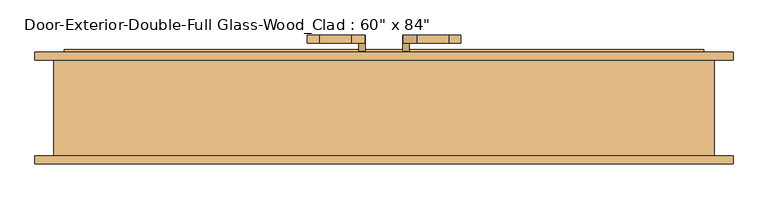
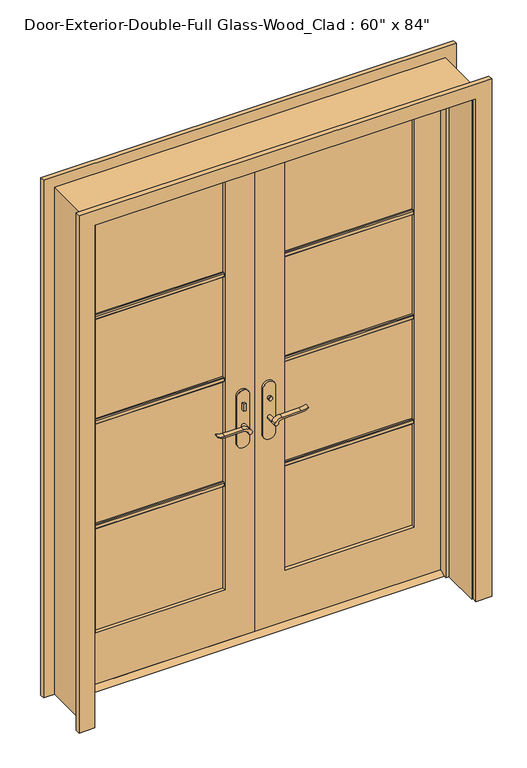
"""IFC4 building model written with IfcOpenShell, lengths in millimetres: door geometry."""

from ifc_helpers import new_model, si_unit, point, frame, frame_2d, origin, place, context, project, spatial, polyline, circle_curve, trimmed, segment, composite_curve, outline, extrude, faceted_brep, source, transform, mapped, element, save


def door_014e9f54(model_context):
    return source(origin(), model_context, "Body", "SolidModel", [
        extrude(outline(polyline([(76.2, 12.7), (111.125, 12.7), (136.525, 0.0), (50.8, 0.0), (76.2, 12.7)])), frame((-762.0, 0.0, 0.0), z_axis=(1.0, 0.0, 0.0), x_axis=(0.0, 1.0, 0.0)), (0.0, 0.0, 1.0), 1524.0),
        extrude(outline(polyline([(-47.4019111, 56.2), (-57.4019111, 56.2), (-57.4019111, 66.2), (-47.4019111, 66.2), (-47.4019111, 56.2)])), frame((0.0, 0.0, 981.9), z_axis=(0.0, 0.0, 1.0), x_axis=(1.0, 0.0, 0.0)), (0.0, 0.0, 1.0), 30.0),
        extrude(outline(composite_curve([segment(trimmed(circle_curve(frame_2d((996.9, -52.4019111)), 8.0), [point((996.9, -60.4019111))], [point((996.9, -44.4019111))], False, "CARTESIAN"), True, "CONTINUOUS"), segment(trimmed(circle_curve(frame_2d((996.9, -52.4019111)), 8.0), [point((996.9, -44.4019111))], [point((996.9, -60.4019111))], False, "CARTESIAN"), True, "CONTINUOUS")], self_intersect=False)), frame((0.0, 121.125, 0.0), z_axis=(0.0, 1.0, 0.0), x_axis=(0.0, 0.0, 1.0)), (0.0, 0.0, 1.0), 10.0),
        extrude(outline(composite_curve([segment(trimmed(circle_curve(frame_2d((897.1555521, -76.0694241)), 37.2832219), [point((919.0523287, -45.8937749))], [point((934.4, -77.7693445))], False, "CARTESIAN"), True, "CONTINUOUS"), segment(polyline([(934.4, -77.7693445), (934.4, -154.045502)]), True, "CONTINUOUS"), segment(trimmed(circle_curve(frame_2d((1017.6850638, -153.9791202)), 83.2850902), [point((934.4, -154.045502))], [point((939.4, -182.4019111))], True, "CARTESIAN"), True, "CONTINUOUS"), segment(polyline([(939.4, -182.4019111), (936.6135558, -182.4019111)]), True, "CONTINUOUS"), segment(trimmed(circle_curve(frame_2d((986.6709207, -150.4622499)), 59.3791355), [point((936.6135558, -182.4019111))], [point((927.4, -154.045502))], False, "CARTESIAN"), True, "CONTINUOUS"), segment(polyline([(927.4, -154.045502), (927.4, -77.7881013)]), True, "CONTINUOUS"), segment(trimmed(circle_curve(frame_2d((909.2738613, -77.7881013)), 18.1261387), [point((927.4, -77.7881013))], [point((914.4, -60.4019111))], True, "CARTESIAN"), True, "CONTINUOUS"), segment(trimmed(circle_curve(frame_2d((914.4, -52.4019111)), 8.0), [point((914.4, -60.4019111))], [point((919.0523287, -45.8937749))], False, "CARTESIAN"), True, "CONTINUOUS")], self_intersect=False)), frame((0.0, 16.2, 0.0), z_axis=(0.0, 1.0, 0.0), x_axis=(0.0, 0.0, 1.0)), (0.0, 0.0, 1.0), 20.0),
        extrude(outline(composite_curve([segment(trimmed(circle_curve(frame_2d((914.4, -52.4019111)), 8.0), [point((914.3999903, -60.4019111))], [point((919.0523287, -45.8937749))], False, "CARTESIAN"), True, "CONTINUOUS"), segment(trimmed(circle_curve(frame_2d((897.1555521, -76.0694241)), 37.2832219), [point((919.0523287, -45.8937749))], [point((934.4, -77.7693445))], False, "CARTESIAN"), True, "CONTINUOUS"), segment(polyline([(934.4, -77.7693445), (934.4, -154.045502)]), True, "CONTINUOUS"), segment(trimmed(circle_curve(frame_2d((1017.6850638, -153.9791202)), 83.2850902), [point((934.4, -154.045502))], [point((939.4, -182.4019111))], True, "CARTESIAN"), True, "CONTINUOUS"), segment(polyline([(939.4, -182.4019111), (936.6135558, -182.4019111)]), True, "CONTINUOUS"), segment(trimmed(circle_curve(frame_2d((986.6709207, -150.4622499)), 59.3791355), [point((936.6135558, -182.4019111))], [point((927.4, -154.045502))], False, "CARTESIAN"), True, "CONTINUOUS"), segment(polyline([(927.4, -154.045502), (927.4, -77.788099)]), True, "CONTINUOUS"), segment(trimmed(circle_curve(frame_2d((909.2738682, -77.788099)), 18.1261318), [point((927.4, -77.788099))], [point((914.3999903, -60.4019111))], True, "CARTESIAN"), True, "CONTINUOUS")], self_intersect=False)), frame((0.0, 151.125, 0.0), z_axis=(0.0, 1.0, 0.0), x_axis=(0.0, 0.0, 1.0)), (0.0, 0.0, 1.0), 20.0),
        extrude(outline(composite_curve([segment(trimmed(circle_curve(frame_2d((914.4, -52.4019111)), 8.0), [point((914.4, -60.4019111))], [point((914.4, -44.4019111))], False, "CARTESIAN"), True, "CONTINUOUS"), segment(trimmed(circle_curve(frame_2d((914.4, -52.4019111)), 8.0), [point((914.4, -44.4019111))], [point((914.4, -60.4019111))], False, "CARTESIAN"), True, "CONTINUOUS")], self_intersect=False)), frame((0.0, 36.2, 0.0), z_axis=(0.0, 1.0, 0.0), x_axis=(0.0, 0.0, 1.0)), (0.0, 0.0, 1.0), 30.0),
        extrude(outline(composite_curve([segment(trimmed(circle_curve(frame_2d((914.4, -52.4019111)), 8.0), [point((914.4, -60.4019111))], [point((914.4, -44.4019111))], False, "CARTESIAN"), True, "CONTINUOUS"), segment(trimmed(circle_curve(frame_2d((914.4, -52.4019111)), 8.0), [point((914.4, -44.4019111))], [point((914.4, -60.4019111))], False, "CARTESIAN"), True, "CONTINUOUS")], self_intersect=False)), frame((0.0, 121.125, 0.0), z_axis=(0.0, 1.0, 0.0), x_axis=(0.0, 0.0, 1.0)), (0.0, 0.0, 1.0), 30.0),
        extrude(outline(composite_curve([segment(polyline([(844.4, -27.4019111), (1039.4, -27.4019111)]), True, "CONTINUOUS"), segment(trimmed(circle_curve(frame_2d((1039.4, -52.4019111)), 25.0), [point((1039.4, -27.4019111))], [point((1039.4, -77.4019111))], False, "CARTESIAN"), True, "CONTINUOUS"), segment(polyline([(1039.4, -77.4019111), (844.4, -77.4019111)]), True, "CONTINUOUS"), segment(trimmed(circle_curve(frame_2d((844.4, -52.4019111)), 25.0), [point((844.4, -77.4019111))], [point((844.4, -27.4019111))], False, "CARTESIAN"), True, "CONTINUOUS")], self_intersect=False)), frame((0.0, 66.2, 0.0), z_axis=(0.0, 1.0, 0.0), x_axis=(0.0, 0.0, 1.0)), (0.0, 0.0, 1.0), 10.0),
        extrude(outline(composite_curve([segment(polyline([(844.4, -27.4019111), (1039.4, -27.4019111)]), True, "CONTINUOUS"), segment(trimmed(circle_curve(frame_2d((1039.4, -52.4019111)), 25.0), [point((1039.4, -27.4019111))], [point((1039.4, -77.4019111))], False, "CARTESIAN"), True, "CONTINUOUS"), segment(polyline([(1039.4, -77.4019111), (844.4, -77.4019111)]), True, "CONTINUOUS"), segment(trimmed(circle_curve(frame_2d((844.4, -52.4019111)), 25.0), [point((844.4, -77.4019111))], [point((844.4, -27.4019111))], False, "CARTESIAN"), True, "CONTINUOUS")], self_intersect=False)), frame((0.0, 111.125, 0.0), z_axis=(0.0, 1.0, 0.0), x_axis=(0.0, 0.0, 1.0)), (0.0, 0.0, 1.0), 10.0),
        extrude(outline(polyline([(47.3875, 131.125), (57.3875, 131.125), (57.3875, 121.125), (47.3875, 121.125), (47.3875, 131.125)])), frame((0.0, 0.0, 981.9), z_axis=(0.0, 0.0, 1.0), x_axis=(1.0, 0.0, 0.0)), (0.0, 0.0, 1.0), 30.0),
        extrude(outline(composite_curve([segment(trimmed(circle_curve(frame_2d((996.9, 52.3875)), 8.0), [point((996.9, 60.3875))], [point((996.9, 44.3875))], False, "CARTESIAN"), True, "CONTINUOUS"), segment(trimmed(circle_curve(frame_2d((996.9, 52.3875)), 8.0), [point((996.9, 44.3875))], [point((996.9, 60.3875))], False, "CARTESIAN"), True, "CONTINUOUS")], self_intersect=False)), frame((0.0, 56.2, 0.0), z_axis=(0.0, 1.0, 0.0), x_axis=(0.0, 0.0, 1.0)), (0.0, 0.0, 1.0), 10.0),
        extrude(outline(composite_curve([segment(trimmed(circle_curve(frame_2d((914.4, 52.3875)), 8.0), [point((919.0523287, 45.8793637))], [point((914.4, 60.3875))], False, "CARTESIAN"), True, "CONTINUOUS"), segment(trimmed(circle_curve(frame_2d((909.2738613, 77.7736901)), 18.1261387), [point((914.4, 60.3875))], [point((927.4, 77.7736901))], True, "CARTESIAN"), True, "CONTINUOUS"), segment(polyline([(927.4, 77.7736901), (927.4, 154.0310909)]), True, "CONTINUOUS"), segment(trimmed(circle_curve(frame_2d((986.6709207, 150.4478388)), 59.3791355), [point((927.4, 154.0310909))], [point((936.6135558, 182.3875))], False, "CARTESIAN"), True, "CONTINUOUS"), segment(polyline([(936.6135558, 182.3875), (939.4, 182.3875)]), True, "CONTINUOUS"), segment(trimmed(circle_curve(frame_2d((1017.6850638, 153.9647091)), 83.2850902), [point((939.4, 182.3875))], [point((934.4, 154.0310909))], True, "CARTESIAN"), True, "CONTINUOUS"), segment(polyline([(934.4, 154.0310909), (934.4, 77.7549333)]), True, "CONTINUOUS"), segment(trimmed(circle_curve(frame_2d((897.1555521, 76.0550129)), 37.2832219), [point((934.4, 77.7549333))], [point((919.0523287, 45.8793637))], False, "CARTESIAN"), True, "CONTINUOUS")], self_intersect=False)), frame((0.0, 151.125, 0.0), z_axis=(0.0, 1.0, 0.0), x_axis=(0.0, 0.0, 1.0)), (0.0, 0.0, 1.0), 20.0),
        extrude(outline(composite_curve([segment(trimmed(circle_curve(frame_2d((909.2738682, 77.7736878)), 18.1261318), [point((914.3999903, 60.3875))], [point((927.4, 77.7736878))], True, "CARTESIAN"), True, "CONTINUOUS"), segment(polyline([(927.4, 77.7736878), (927.4, 154.0310909)]), True, "CONTINUOUS"), segment(trimmed(circle_curve(frame_2d((986.6709207, 150.4478388)), 59.3791355), [point((927.4, 154.0310909))], [point((936.6135558, 182.3875))], False, "CARTESIAN"), True, "CONTINUOUS"), segment(polyline([(936.6135558, 182.3875), (939.4, 182.3875)]), True, "CONTINUOUS"), segment(trimmed(circle_curve(frame_2d((1017.6850638, 153.9647091)), 83.2850902), [point((939.4, 182.3875))], [point((934.4, 154.0310909))], True, "CARTESIAN"), True, "CONTINUOUS"), segment(polyline([(934.4, 154.0310909), (934.4, 77.7549333)]), True, "CONTINUOUS"), segment(trimmed(circle_curve(frame_2d((897.1555521, 76.0550129)), 37.2832219), [point((934.4, 77.7549333))], [point((919.0523287, 45.8793637))], False, "CARTESIAN"), True, "CONTINUOUS"), segment(trimmed(circle_curve(frame_2d((914.4, 52.3875)), 8.0), [point((919.0523287, 45.8793637))], [point((914.3999903, 60.3875))], False, "CARTESIAN"), True, "CONTINUOUS")], self_intersect=False)), frame((0.0, 16.2, 0.0), z_axis=(0.0, 1.0, 0.0), x_axis=(0.0, 0.0, 1.0)), (0.0, 0.0, 1.0), 20.0),
        extrude(outline(composite_curve([segment(trimmed(circle_curve(frame_2d((914.4, 52.3875)), 8.0), [point((914.4, 60.3875))], [point((914.4, 44.3875))], False, "CARTESIAN"), True, "CONTINUOUS"), segment(trimmed(circle_curve(frame_2d((914.4, 52.3875)), 8.0), [point((914.4, 44.3875))], [point((914.4, 60.3875))], False, "CARTESIAN"), True, "CONTINUOUS")], self_intersect=False)), frame((0.0, 121.125, 0.0), z_axis=(0.0, 1.0, 0.0), x_axis=(0.0, 0.0, 1.0)), (0.0, 0.0, 1.0), 30.0),
        extrude(outline(composite_curve([segment(trimmed(circle_curve(frame_2d((914.4, 52.3875)), 8.0), [point((914.4, 60.3875))], [point((914.4, 44.3875))], False, "CARTESIAN"), True, "CONTINUOUS"), segment(trimmed(circle_curve(frame_2d((914.4, 52.3875)), 8.0), [point((914.4, 44.3875))], [point((914.4, 60.3875))], False, "CARTESIAN"), True, "CONTINUOUS")], self_intersect=False)), frame((0.0, 36.2, 0.0), z_axis=(0.0, 1.0, 0.0), x_axis=(0.0, 0.0, 1.0)), (0.0, 0.0, 1.0), 30.0),
        extrude(outline(composite_curve([segment(trimmed(circle_curve(frame_2d((844.4, 52.3875)), 25.0), [point((844.4, 27.3875))], [point((844.4, 77.3875))], False, "CARTESIAN"), True, "CONTINUOUS"), segment(polyline([(844.4, 77.3875), (1039.4, 77.3875)]), True, "CONTINUOUS"), segment(trimmed(circle_curve(frame_2d((1039.4, 52.3875)), 25.0), [point((1039.4, 77.3875))], [point((1039.4, 27.3875))], False, "CARTESIAN"), True, "CONTINUOUS"), segment(polyline([(1039.4, 27.3875), (844.4, 27.3875)]), True, "CONTINUOUS")], self_intersect=False)), frame((0.0, 111.125, 0.0), z_axis=(0.0, 1.0, 0.0), x_axis=(0.0, 0.0, 1.0)), (0.0, 0.0, 1.0), 10.0),
        extrude(outline(composite_curve([segment(trimmed(circle_curve(frame_2d((844.4, 52.3875)), 25.0), [point((844.4, 27.3875))], [point((844.4, 77.3875))], False, "CARTESIAN"), True, "CONTINUOUS"), segment(polyline([(844.4, 77.3875), (1039.4, 77.3875)]), True, "CONTINUOUS"), segment(trimmed(circle_curve(frame_2d((1039.4, 52.3875)), 25.0), [point((1039.4, 77.3875))], [point((1039.4, 27.3875))], False, "CARTESIAN"), True, "CONTINUOUS"), segment(polyline([(1039.4, 27.3875), (844.4, 27.3875)]), True, "CONTINUOUS")], self_intersect=False)), frame((0.0, 66.2, 0.0), z_axis=(0.0, 1.0, 0.0), x_axis=(0.0, 0.0, 1.0)), (0.0, 0.0, 1.0), 10.0),
        extrude(outline(polyline([(90.17, 1578.371875), (90.17, 1559.321875), (83.82, 1559.321875), (80.645, 1562.496875), (80.645, 1575.196875), (83.82, 1578.371875), (90.17, 1578.371875)])), frame((120.65, 0.0, 0.0), z_axis=(1.0, 0.0, 0.0), x_axis=(0.0, 1.0, 0.0)), (0.0, 0.0, 1.0), 520.7),
        extrude(outline(polyline([(90.17, 1132.68125), (90.17, 1113.63125), (83.82, 1113.63125), (80.645, 1116.80625), (80.645, 1129.50625), (83.82, 1132.68125), (90.17, 1132.68125)])), frame((120.65, 0.0, 0.0), z_axis=(1.0, 0.0, 0.0), x_axis=(0.0, 1.0, 0.0)), (0.0, 0.0, 1.0), 520.7),
        extrude(outline(polyline([(90.17, 686.990625), (90.17, 667.940625), (83.82, 667.940625), (80.645, 671.115625), (80.645, 683.815625), (83.82, 686.990625), (90.17, 686.990625)])), frame((120.65, 0.0, 0.0), z_axis=(1.0, 0.0, 0.0), x_axis=(0.0, 1.0, 0.0)), (0.0, 0.0, 1.0), 520.7),
        extrude(outline(polyline([(97.155, 1578.371875), (103.505, 1578.371875), (106.68, 1575.196875), (106.68, 1562.496875), (103.505, 1559.321875), (97.155, 1559.321875), (97.155, 1578.371875)])), frame((-641.35, 0.0, 0.0), z_axis=(1.0, 0.0, 0.0), x_axis=(0.0, 1.0, 0.0)), (0.0, 0.0, 1.0), 520.7),
        extrude(outline(polyline([(97.155, 1132.68125), (103.505, 1132.68125), (106.68, 1129.50625), (106.68, 1116.80625), (103.505, 1113.63125), (97.155, 1113.63125), (97.155, 1132.68125)])), frame((-641.35, 0.0, 0.0), z_axis=(1.0, 0.0, 0.0), x_axis=(0.0, 1.0, 0.0)), (0.0, 0.0, 1.0), 520.7),
        extrude(outline(polyline([(97.155, 686.990625), (103.505, 686.990625), (106.68, 683.815625), (106.68, 671.115625), (103.505, 667.940625), (97.155, 667.940625), (97.155, 686.990625)])), frame((-641.35, 0.0, 0.0), z_axis=(1.0, 0.0, 0.0), x_axis=(0.0, 1.0, 0.0)), (0.0, 0.0, 1.0), 520.7),
        extrude(outline(polyline([(97.155, 1578.371875), (103.505, 1578.371875), (106.68, 1575.196875), (106.68, 1562.496875), (103.505, 1559.321875), (97.155, 1559.321875), (97.155, 1578.371875)])), frame((120.65, 0.0, 0.0), z_axis=(1.0, 0.0, 0.0), x_axis=(0.0, 1.0, 0.0)), (0.0, 0.0, 1.0), 520.7),
        extrude(outline(polyline([(97.155, 1132.68125), (103.505, 1132.68125), (106.68, 1129.50625), (106.68, 1116.80625), (103.505, 1113.63125), (97.155, 1113.63125), (97.155, 1132.68125)])), frame((120.65, 0.0, 0.0), z_axis=(1.0, 0.0, 0.0), x_axis=(0.0, 1.0, 0.0)), (0.0, 0.0, 1.0), 520.7),
        extrude(outline(polyline([(97.155, 686.990625), (103.505, 686.990625), (106.68, 683.815625), (106.68, 671.115625), (103.505, 667.940625), (97.155, 667.940625), (97.155, 686.990625)])), frame((120.65, 0.0, 0.0), z_axis=(1.0, 0.0, 0.0), x_axis=(0.0, 1.0, 0.0)), (0.0, 0.0, 1.0), 520.7),
        extrude(outline(polyline([(90.17, 1578.371875), (90.17, 1559.321875), (83.82, 1559.321875), (80.645, 1562.496875), (80.645, 1575.196875), (83.82, 1578.371875), (90.17, 1578.371875)])), frame((-641.35, 0.0, 0.0), z_axis=(1.0, 0.0, 0.0), x_axis=(0.0, 1.0, 0.0)), (0.0, 0.0, 1.0), 520.7),
        extrude(outline(polyline([(90.17, 1132.68125), (90.17, 1113.63125), (83.82, 1113.63125), (80.645, 1116.80625), (80.645, 1129.50625), (83.82, 1132.68125), (90.17, 1132.68125)])), frame((-641.35, 0.0, 0.0), z_axis=(1.0, 0.0, 0.0), x_axis=(0.0, 1.0, 0.0)), (0.0, 0.0, 1.0), 520.7),
        extrude(outline(polyline([(90.17, 686.990625), (90.17, 667.940625), (83.82, 667.940625), (80.645, 671.115625), (80.645, 683.815625), (83.82, 686.990625), (90.17, 686.990625)])), frame((-641.35, 0.0, 0.0), z_axis=(1.0, 0.0, 0.0), x_axis=(0.0, 1.0, 0.0)), (0.0, 0.0, 1.0), 520.7),
        extrude(outline(polyline([(0.0, 768.35), (0.0, 831.85), (2203.45, 831.85), (2203.45, -831.85), (0.0, -831.85), (0.0, -768.35), (2139.95, -768.35), (2139.95, 768.35), (0.0, 768.35)])), frame((0.0, 111.125, 0.0), z_axis=(0.0, 1.0, 0.0), x_axis=(0.0, 0.0, 1.0)), (0.0, 0.0, 1.0), 19.05),
        extrude(outline(polyline([(0.0, 768.35), (0.0, 831.85), (2203.45, 831.85), (2203.45, -831.85), (0.0, -831.85), (0.0, -768.35), (2139.95, -768.35), (2139.95, 768.35), (0.0, 768.35)])), frame((0.0, -136.525, 0.0), z_axis=(0.0, 1.0, 0.0), x_axis=(0.0, 0.0, 1.0)), (0.0, 0.0, 1.0), 19.05),
        extrude(outline(polyline([(12.7, 762.0), (2133.6, 762.0), (2133.6, 1.5875), (12.7, 1.5875), (12.7, 762.0)]), holes=[polyline([(2014.5375, 120.65), (2014.5375, 641.35), (231.775, 641.35), (231.775, 120.65), (2014.5375, 120.65)])]), frame((0.0, 76.2, 0.0), z_axis=(0.0, 1.0, 0.0), x_axis=(0.0, 0.0, 1.0)), (0.0, 0.0, 1.0), 34.925),
        extrude(outline(polyline([(2133.6, -762.0), (12.7, -762.0), (12.7, -1.6019111), (2133.6, -1.6019111), (2133.6, -762.0)]), holes=[polyline([(231.775, -641.35), (2014.5375, -641.35), (2014.5375, -120.65), (231.775, -120.65), (231.775, -641.35)])]), frame((0.0, 76.2, 0.0), z_axis=(0.0, 1.0, 0.0), x_axis=(0.0, 0.0, 1.0)), (0.0, 0.0, 1.0), 34.925),
        faceted_brep([(787.4, 111.125, 0.0), (787.4, -117.475, 0.0), (762.0, -117.475, 0.0), (762.0, 41.275, 0.0), (749.3, 41.275, 0.0), (749.3, 76.2, 0.0), (762.0, 76.2, 0.0), (762.0, 111.125, 0.0), (787.4, 111.125, 2159.0), (787.4, -117.475, 2159.0), (-787.4, -117.475, 2159.0), (-787.4, -117.475, 0.0), (-762.0, -117.475, 0.0), (-762.0, -117.475, 2133.6), (762.0, -117.475, 2133.6), (762.0, 41.275, 2133.6), (-762.0, 41.275, 2133.6), (-762.0, 41.275, 0.0), (-749.3, 41.275, 0.0), (-749.3, 41.275, 2120.9), (749.3, 41.275, 2120.9), (749.3, 76.2, 2120.9), (1.5875, 76.2, 2120.9), (-1.6019111, 76.2, 2120.9), (-749.3, 76.2, 2120.9), (-749.3, 76.2, 0.0), (-762.0, 76.2, 0.0), (-762.0, 76.2, 2133.6), (-1.6019111, 76.2, 2133.6), (1.5875, 76.2, 2133.6), (762.0, 76.2, 2133.6), (762.0, 111.125, 2133.6), (1.5875, 111.125, 2133.6), (-1.6019111, 111.125, 2133.6), (-762.0, 111.125, 2133.6), (-762.0, 111.125, 0.0), (-787.4, 111.125, 0.0), (-787.4, 111.125, 2159.0)], [[[0, 1, 2, 3, 4, 5, 6, 7]], [[1, 0, 8, 9]], [[2, 1, 9, 10, 11, 12, 13, 14]], [[3, 2, 14, 15]], [[4, 3, 15, 16, 17, 18, 19, 20]], [[5, 4, 20, 21]], [[6, 5, 21, 22, 23, 24, 25, 26, 27, 28, 29, 30]], [[7, 6, 30, 31]], [[0, 7, 31, 32, 33, 34, 35, 36, 37, 8]], [[9, 8, 37, 10]], [[14, 13, 16, 15]], [[20, 19, 24, 23, 22, 21]], [[31, 30, 29, 28, 27, 34, 33, 32]], [[12, 11, 36, 35, 26, 25, 18, 17]], [[11, 10, 37, 36]], [[13, 12, 17, 16]], [[19, 18, 25, 24]], [[27, 26, 35, 34]]]),
        extrude(outline(polyline([(641.35, 90.17), (120.65, 90.17), (120.65, 97.155), (641.35, 97.155), (641.35, 90.17)])), frame((0.0, 0.0, 231.775), z_axis=(0.0, 0.0, 1.0), x_axis=(1.0, 0.0, 0.0)), (0.0, 0.0, 1.0), 1782.7625),
        extrude(outline(polyline([(-120.65, 90.17), (-641.35, 90.17), (-641.35, 97.155), (-120.65, 97.155), (-120.65, 90.17)])), frame((0.0, 0.0, 231.775), z_axis=(0.0, 0.0, 1.0), x_axis=(1.0, 0.0, 0.0)), (0.0, 0.0, 1.0), 1782.7625),
    ])


if __name__ == "__main__":
    model = new_model("IFC4")
    model_context = context("Model", 3, world=origin())
    ifc_project = project(units=[si_unit("LENGTHUNIT", "METRE", prefix="MILLI")], contexts=[model_context])
    site = spatial("IfcSite", under=ifc_project)
    building = spatial("IfcBuilding", under=site)
    placement = place(None, origin())
    door_shape = door_014e9f54(model_context)
    element("IfcDoor", 1, ObjectType="Door-Exterior-Double-Full Glass-Wood_Clad : 60\" x 84\"", at=placement, inside=building, context=model_context, shape_type="MappedRepresentation", body=[
        mapped(door_shape, transform((0.0, 0.0, 0.0), x_axis=(1.0, 0.0, 0.0), y_axis=(0.0, 1.0, 0.0), z_axis=(0.0, 0.0, 1.0))),
    ])
    save(model, "model.ifc")

# Revit data of these elements
# Type "Door-Exterior-Double-Full Glass-Wood_Clad : 60\" x 84\""
#   Type Mark = "9"
#   Assembly Code = "B2030100"
#   Analytic Construction = "French door, wood frame with double glass"
#   Top Rail = 0' - 4 11/16"
#   Threshold Offset [instance default] = 0' - 0 1/2"
#   Thickness = 0' - 1 3/8"
#   Thermal Resistance (R) = 1.9158 (h·ft²·°F)/BTU
#   Swing Angle [instance default] = 90.00°
#   Stiles = 0' - 4 3/4"
#   Rough Width = 5' - 2"
#   Rough Height = 7' - 1"
#   Panel Width = 2' - 6"
#   Door Offset [instance default] = 0' - 0"
#   Height = 7' - 0"
#   Width = 5' - 0"
#   Heat Transfer Coefficient (U) = 0.5220 BTU/(h·ft²·°F)
#   Bottom Rail = 0' - 9 1/8"
#   Exterior Trim [instance default] = yes
#   Threshold [instance default] = yes
#   Show Grill [instance default] = yes
#   Function = 1
#   Trim Material = Cherry
#   Threshold Material = Cherry
#   Panel Material = Cherry
#   Glazing = Glass
#   Frame Material = Cherry
#   Door Handle Material = Aluminum
#   Visual Light Transmittance = 0
#   Solar Heat Gain Coefficient = 0
#   Wall Closure = (empty or 0)
#   Construction Type = (empty or 0)
# Element 1 (IfcDoor, "Door-Exterior-Double-Full Glass-Wood_Clad : 60\" x 84\"")
#   Materials on its faces: "Cherry", "Aluminum", "Glass"
# Materials
#   "Cherry": class "Wood", colour RGB 226 177 128, transparency 0, Description = "Prunus Serotina", Cost = 0
#   "Glass": class "Glass", colour RGB 0 128 192, transparency 0.75, Description = "Soda Lime Glass", Cost = 0
#   "Aluminum": class "Metal", colour RGB 247 247 247, transparency 0, Description = "Aluminum 6061", Cost = 0
